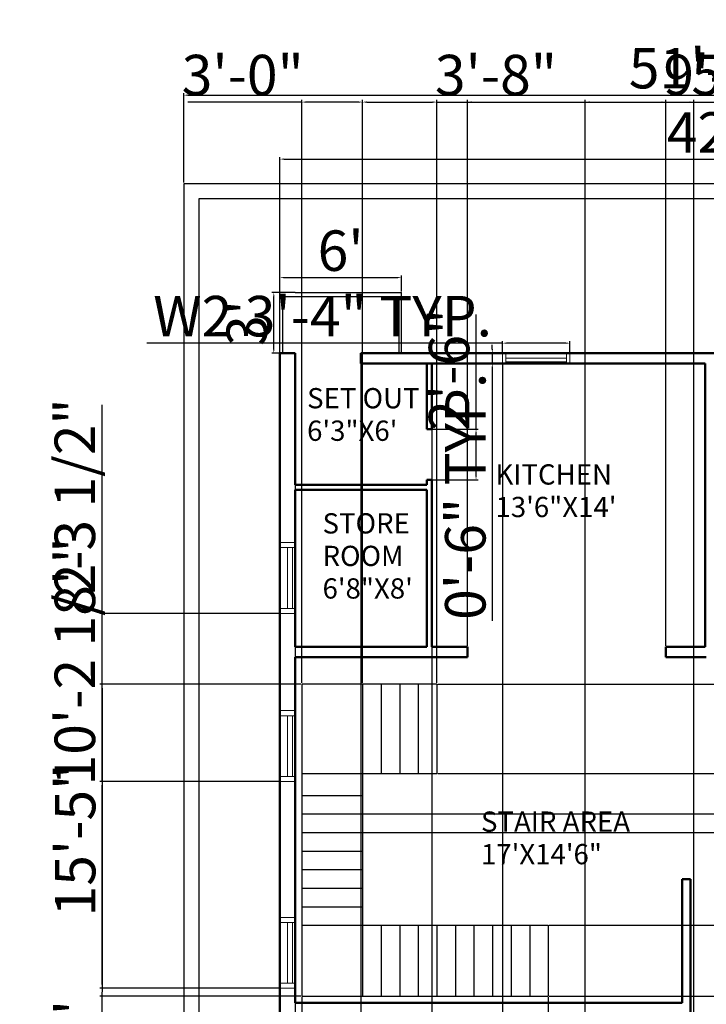
# Model space of a CAD drawing. Units: inches. Extents: x 2047 to 3023, y 479 to 1545.
# Tile 2 of 3: x 2047 to 2454, y 961 to 1545. Entities that reach past the tile are written whole.
import ezdxf

# ---------------------------------------------------------------- set-up
doc = ezdxf.new("R2010")
doc.units = ezdxf.units.IN
for name, color, linetype, lineweight in [('A-ANNO-DIMS', 2, 'Continuous', 18), ('A-AREA-IDEN', 7, 'Continuous', 25), ('A-FLOR', 8, 'Continuous', 25), ('A-FLOR-STRS', 7, 'Continuous', 25), ('A-GLAZ', 4, 'Continuous', 18), ('A-WALL', 7, 'Continuous', 50), ('C-PROP', 8, 'Continuous', 30)]:
    doc.layers.add(name, color=color, linetype=linetype, lineweight=lineweight)
doc.styles.get("Standard").update_dxf_attribs({"font": 'arial.ttf'})
doc.dimstyles.new('ISO-25', dxfattribs={"dimtxt": 24, "dimasz": 2.5, "dimexe": 1.25, "dimexo": 0.625, "dimtad": 1, "dimdec": 1, "dimlunit": 3, "dimtxsty": 'Standard', "dimcen": 2.5, "dimadec": 0, "dimazin": 0, "dimtfac": 1, "dimtdec": 1, "dimtmove": 0, "dimatfit": 3, "dimfxl": 1, "dimarcsym": 0})

# ---------------------------------------------------------------- blocks, each defined once
blk = doc.blocks.new('*D1')
at = {"layer": 'A-ANNO-DIMS', "color": 0, "lineweight": -2, "transparency": 16777216}
for p, q in [((2200.28, 1382.98), (2196.04, 1382.98)), ((2197.29, 1349.48), (2197.29, 1380.48)), ((2200.28, 1346.98), (2196.04, 1346.98))]:
    blk.add_line(p, q, dxfattribs=at)
at = {"layer": 'A-ANNO-DIMS', "color": 0, "transparency": 16777216}
for points in [[(2196.87, 1380.48), (2197.7, 1380.48), (2197.29, 1382.98)], [(2196.87, 1349.48), (2197.7, 1349.48), (2197.29, 1346.98)]]:
    blk.add_solid(points, dxfattribs=at)
at = {"layer": 'Defpoints', "color": 0, "transparency": 16777216}
for p in [(2197.29, 1382.98), (2200.91, 1382.98), (2200.91, 1346.98)]:
    blk.add_point(p, dxfattribs=at)
at = {"layer": 'A-ANNO-DIMS', "color": 0, "transparency": 16777216, "insert": (2184.4, 1364.98), "char_height": 24, "attachment_point": 5, "rotation": 90}
blk.add_mtext("3'", dxfattribs=at)
blk = doc.blocks.new('*D2')
at = {"layer": 'A-ANNO-DIMS', "color": 0, "lineweight": -2, "transparency": 16777216}
for p, q in [((2200.91, 1383.61), (2200.91, 1393.05)), ((2203.41, 1391.8), (2270.41, 1391.8)), ((2272.91, 1383.61), (2272.91, 1393.05))]:
    blk.add_line(p, q, dxfattribs=at)
at = {"layer": 'A-ANNO-DIMS', "color": 0, "transparency": 16777216}
for points in [[(2203.41, 1392.22), (2203.41, 1391.39), (2200.91, 1391.8)], [(2270.41, 1392.22), (2270.41, 1391.39), (2272.91, 1391.8)]]:
    blk.add_solid(points, dxfattribs=at)
at = {"layer": 'Defpoints', "color": 0, "transparency": 16777216}
for p in [(2272.91, 1391.8), (2200.91, 1382.98), (2272.91, 1382.98)]:
    blk.add_point(p, dxfattribs=at)
at = {"layer": 'A-ANNO-DIMS', "color": 0, "transparency": 16777216, "insert": (2236.91, 1404.68), "char_height": 24, "attachment_point": 5}
blk.add_mtext("6'", dxfattribs=at)
blk = doc.blocks.new('*D4')
at = {"layer": 'A-ANNO-DIMS', "color": 0, "lineweight": -2, "transparency": 16777216}
for p, q in [((2143.91, 1448.11), (2143.91, 1501.19)), ((2146.41, 1499.94), (2759.41, 1499.94)), ((2761.91, 1448.11), (2761.91, 1501.19))]:
    blk.add_line(p, q, dxfattribs=at)
at = {"layer": 'A-ANNO-DIMS', "color": 0, "transparency": 16777216}
for points in [[(2146.41, 1500.36), (2146.41, 1499.52), (2143.91, 1499.94)], [(2759.41, 1500.36), (2759.41, 1499.52), (2761.91, 1499.94)]]:
    blk.add_solid(points, dxfattribs=at)
at = {"layer": 'Defpoints', "color": 0, "transparency": 16777216}
for p in [(2761.91, 1499.94), (2143.91, 1447.48), (2761.91, 1447.48)]:
    blk.add_point(p, dxfattribs=at)
at = {"layer": 'A-ANNO-DIMS', "color": 0, "transparency": 16777216, "insert": (2452.91, 1512.82), "char_height": 24, "attachment_point": 5}
blk.add_mtext('51\'-6"', dxfattribs=at)
blk = doc.blocks.new('*D5')
at = {"layer": 'A-ANNO-DIMS', "color": 0, "lineweight": -2, "transparency": 16777216}
for p, q in [((2200.91, 1347.61), (2200.91, 1463.28)), ((2203.41, 1462.03), (2702.41, 1462.03)), ((2704.91, 1347.61), (2704.91, 1463.28))]:
    blk.add_line(p, q, dxfattribs=at)
at = {"layer": 'A-ANNO-DIMS', "color": 0, "transparency": 16777216}
for points in [[(2203.41, 1462.44), (2203.41, 1461.61), (2200.91, 1462.03)], [(2702.41, 1462.44), (2702.41, 1461.61), (2704.91, 1462.03)]]:
    blk.add_solid(points, dxfattribs=at)
at = {"layer": 'Defpoints', "color": 0, "transparency": 16777216}
for p in [(2704.91, 1462.03), (2200.91, 1346.98), (2704.91, 1346.98)]:
    blk.add_point(p, dxfattribs=at)
at = {"layer": 'A-ANNO-DIMS', "color": 0, "transparency": 16777216, "insert": (2452.91, 1474.7), "char_height": 24, "attachment_point": 5}
blk.add_mtext("42'", dxfattribs=at)
blk = doc.blocks.new('*D10')
at = {"layer": 'A-ANNO-DIMS', "color": 0, "lineweight": -2, "transparency": 16777216}
for p, q in [((2317.13, 1301.98), (2317.13, 1369.94)), ((2291.53, 1301.98), (2318.38, 1301.98)), ((2317.13, 1274.48), (2317.13, 1299.48)), ((2291.53, 1271.98), (2318.38, 1271.98))]:
    blk.add_line(p, q, dxfattribs=at)
at = {"layer": 'A-ANNO-DIMS', "color": 0, "transparency": 16777216}
for points in [[(2316.71, 1299.48), (2317.55, 1299.48), (2317.13, 1301.98)], [(2316.71, 1274.48), (2317.55, 1274.48), (2317.13, 1271.98)]]:
    blk.add_solid(points, dxfattribs=at)
at = {"layer": 'Defpoints', "color": 0, "transparency": 16777216}
for p in [(2290.91, 1301.98), (2317.13, 1301.98), (2290.91, 1271.98)]:
    blk.add_point(p, dxfattribs=at)
at = {"layer": 'A-ANNO-DIMS', "color": 0, "transparency": 16777216, "insert": (2304.25, 1337.21), "char_height": 24, "attachment_point": 5, "rotation": 90}
blk.add_mtext('2\'-6"', dxfattribs=at)
blk = doc.blocks.new('WIN-36IN-9IN-FRAME')
for p, q in [((9, 42), (0, 42)), ((9, 39), (0, 39)), ((0, 39), (0, 3)), ((4.5, 3), (4.5, 39)), ((7.5, 3), (7.5, 39)), ((9, 3), (9, 39)), ((0, 3), (9, 3)), ((0, 0), (9, 0))]:
    blk.add_line(p, q)
blk = doc.blocks.new('WIN-36IN-6IN-FRAME')
for p, q in [((0, 6), (0, 0)), ((38, 6), (2, 6)), ((2, 6), (2, 0)), ((38, 0), (38, 6)), ((40, 0), (40, 6)), ((38, 5), (2, 5)), ((38, 3), (2, 3)), ((2, 0), (38, 0))]:
    blk.add_line(p, q)
blk = doc.blocks.new('*D16')
at = {"layer": 'A-ANNO-DIMS', "color": 0, "lineweight": -2, "transparency": 16777216}
for p, q in [((2332.76, 1347.61), (2332.76, 1354.23)), ((2372.76, 1347.61), (2372.76, 1354.23)), ((2332.76, 1352.98), (2122.13, 1352.98)), ((2370.26, 1352.98), (2335.26, 1352.98))]:
    blk.add_line(p, q, dxfattribs=at)
at = {"layer": 'A-ANNO-DIMS', "color": 0, "transparency": 16777216}
for points in [[(2335.26, 1353.4), (2335.26, 1352.56), (2332.76, 1352.98)], [(2370.26, 1353.4), (2370.26, 1352.56), (2372.76, 1352.98)]]:
    blk.add_solid(points, dxfattribs=at)
at = {"layer": 'Defpoints', "color": 0, "transparency": 16777216}
for p in [(2332.76, 1352.98), (2332.76, 1346.98), (2372.76, 1346.98)]:
    blk.add_point(p, dxfattribs=at)
at = {"layer": 'A-ANNO-DIMS', "color": 0, "transparency": 16777216, "insert": (2226.2, 1365.87), "char_height": 24, "attachment_point": 5}
blk.add_mtext('W2 3\'-4" TYP.', dxfattribs=at)
blk = doc.blocks.new('*D17')
at = {"layer": 'A-ANNO-DIMS', "color": 0, "lineweight": -2, "transparency": 16777216}
for p, q in [((2326.76, 1349.48), (2326.76, 1351.98)), ((2332.14, 1346.98), (2325.51, 1346.98)), ((2326.76, 1346.98), (2326.76, 1340.98)), ((2332.14, 1340.98), (2325.51, 1340.98)), ((2326.76, 1338.48), (2326.76, 1188.44))]:
    blk.add_line(p, q, dxfattribs=at)
at = {"layer": 'A-ANNO-DIMS', "color": 0, "transparency": 16777216}
for points in [[(2326.35, 1349.48), (2327.18, 1349.48), (2326.76, 1346.98)], [(2326.35, 1338.48), (2327.18, 1338.48), (2326.76, 1340.98)]]:
    blk.add_solid(points, dxfattribs=at)
at = {"layer": 'Defpoints', "color": 0, "transparency": 16777216}
for p in [(2332.76, 1346.98), (2326.76, 1340.98), (2332.76, 1340.98)]:
    blk.add_point(p, dxfattribs=at)
at = {"layer": 'A-ANNO-DIMS', "color": 0, "transparency": 16777216, "insert": (2313.88, 1262.21), "char_height": 24, "attachment_point": 5, "rotation": 90}
blk.add_mtext('0\'-6" TYP.', dxfattribs=at)
blk = doc.blocks.new('*D29')
at = {"layer": 'A-ANNO-DIMS', "color": 0, "lineweight": -2, "transparency": 16777216}
for p, q in [((2200.28, 970.66), (2094.31, 970.66)), ((2095.56, 887.12), (2095.56, 968.16)), ((2200.28, 884.62), (2094.31, 884.62))]:
    blk.add_line(p, q, dxfattribs=at)
at = {"layer": 'A-ANNO-DIMS', "color": 0, "transparency": 16777216}
for points in [[(2095.14, 968.16), (2095.97, 968.16), (2095.56, 970.66)], [(2095.14, 887.12), (2095.97, 887.12), (2095.56, 884.62)]]:
    blk.add_solid(points, dxfattribs=at)
at = {"layer": 'Defpoints', "color": 0, "transparency": 16777216}
for p in [(2095.56, 970.66), (2200.91, 970.66), (2200.91, 884.62)]:
    blk.add_point(p, dxfattribs=at)
at = {"layer": 'A-ANNO-DIMS', "color": 0, "transparency": 16777216, "insert": (2082.88, 927.64), "char_height": 24, "attachment_point": 5, "rotation": 90}
blk.add_mtext('7\'-2"', dxfattribs=at)
blk = doc.blocks.new('*D30')
at = {"layer": 'A-ANNO-DIMS', "color": 0, "lineweight": -2, "transparency": 16777216}
for p, q in [((2095.56, 1093.2), (2095.56, 1233.06)), ((2200.28, 1093.2), (2094.31, 1093.2)), ((2095.56, 973.16), (2095.56, 1090.7)), ((2200.28, 970.66), (2094.31, 970.66))]:
    blk.add_line(p, q, dxfattribs=at)
at = {"layer": 'A-ANNO-DIMS', "color": 0, "transparency": 16777216}
for points in [[(2095.14, 1090.7), (2095.97, 1090.7), (2095.56, 1093.2)], [(2095.14, 973.16), (2095.97, 973.16), (2095.56, 970.66)]]:
    blk.add_solid(points, dxfattribs=at)
at = {"layer": 'Defpoints', "color": 0, "transparency": 16777216}
for p in [(2095.56, 1093.2), (2200.91, 1093.2), (2200.91, 970.66)]:
    blk.add_point(p, dxfattribs=at)
at = {"layer": 'A-ANNO-DIMS', "color": 0, "transparency": 16777216, "insert": (2082.52, 1164.38), "char_height": 24, "attachment_point": 5, "rotation": 90}
blk.add_mtext('10\'-2 1/2"', dxfattribs=at)
blk = doc.blocks.new('*D31')
at = {"layer": 'A-ANNO-DIMS', "color": 0, "lineweight": -2, "transparency": 16777216}
for p, q in [((2095.56, 1192.82), (2095.56, 1316.32)), ((2200.28, 1192.82), (2094.31, 1192.82)), ((2095.56, 1095.7), (2095.56, 1190.32)), ((2200.28, 1093.2), (2094.31, 1093.2))]:
    blk.add_line(p, q, dxfattribs=at)
at = {"layer": 'A-ANNO-DIMS', "color": 0, "transparency": 16777216}
for points in [[(2095.14, 1190.32), (2095.97, 1190.32), (2095.56, 1192.82)], [(2095.14, 1095.7), (2095.97, 1095.7), (2095.56, 1093.2)]]:
    blk.add_solid(points, dxfattribs=at)
at = {"layer": 'Defpoints', "color": 0, "transparency": 16777216}
for p in [(2095.56, 1192.82), (2200.91, 1192.82), (2200.91, 1093.2)]:
    blk.add_point(p, dxfattribs=at)
at = {"layer": 'A-ANNO-DIMS', "color": 0, "transparency": 16777216, "insert": (2082.52, 1255.82), "char_height": 24, "attachment_point": 5, "rotation": 90}
blk.add_mtext('8\'-3 1/2"', dxfattribs=at)
blk = doc.blocks.new('*D37')
at = {"layer": 'A-ANNO-DIMS', "color": 0, "lineweight": -2, "transparency": 16777216}
for p, q in [((2290.91, 1340.36), (2290.91, 500.88)), ((2332.76, 1340.36), (2332.76, 500.88)), ((2293.41, 502.13), (2330.26, 502.13)), ((2332.76, 502.13), (2400.29, 502.13))]:
    blk.add_line(p, q, dxfattribs=at)
at = {"layer": 'A-ANNO-DIMS', "color": 0, "transparency": 16777216}
for points in [[(2293.41, 502.55), (2293.41, 501.71), (2290.91, 502.13)], [(2330.26, 502.55), (2330.26, 501.71), (2332.76, 502.13)]]:
    blk.add_solid(points, dxfattribs=at)
at = {"layer": 'Defpoints', "color": 0, "transparency": 16777216}
for p in [(2290.91, 1340.98), (2332.76, 1340.98), (2332.76, 502.13)]:
    blk.add_point(p, dxfattribs=at)
at = {"layer": 'A-ANNO-DIMS', "color": 0, "transparency": 16777216, "insert": (2367.78, 515.02), "char_height": 24, "attachment_point": 5}
blk.add_mtext('3\'-6"', dxfattribs=at)
blk = doc.blocks.new('*D41')
at = {"layer": 'A-ANNO-DIMS', "color": 0, "lineweight": -2, "transparency": 16777216}
for p, q in [((2381.88, 867.61), (2381.88, 1497.08)), ((2384.38, 1495.83), (2443.66, 1495.83)), ((2446.16, 867.61), (2446.16, 1497.08)), ((2446.16, 1495.83), (2569.64, 1495.83))]:
    blk.add_line(p, q, dxfattribs=at)
at = {"layer": 'A-ANNO-DIMS', "color": 0, "transparency": 16777216}
for points in [[(2384.38, 1496.25), (2384.38, 1495.41), (2381.88, 1495.83)], [(2443.66, 1496.25), (2443.66, 1495.41), (2446.16, 1495.83)]]:
    blk.add_solid(points, dxfattribs=at)
at = {"layer": 'Defpoints', "color": 0, "transparency": 16777216}
for p in [(2446.16, 1495.83), (2381.88, 866.98), (2446.16, 866.98)]:
    blk.add_point(p, dxfattribs=at)
at = {"layer": 'A-ANNO-DIMS', "color": 0, "transparency": 16777216, "insert": (2509.15, 1508.86), "char_height": 24, "attachment_point": 5}
blk.add_mtext('5\'-4 1/2"', dxfattribs=at)
blk = doc.blocks.new('*D42')
at = {"layer": 'A-ANNO-DIMS', "color": 0, "lineweight": -2, "transparency": 16777216}
for p, q in [((2810.26, 950.97), (2810.26, 1016.25)), ((2362.53, 950.97), (2811.51, 950.97)), ((2810.26, 932.42), (2810.26, 948.47)), ((2362.53, 929.92), (2811.51, 929.92))]:
    blk.add_line(p, q, dxfattribs=at)
at = {"layer": 'A-ANNO-DIMS', "color": 0, "transparency": 16777216}
for points in [[(2809.84, 948.47), (2810.67, 948.47), (2810.26, 950.97)], [(2809.84, 932.42), (2810.67, 932.42), (2810.26, 929.92)]]:
    blk.add_solid(points, dxfattribs=at)
at = {"layer": 'Defpoints', "color": 0, "transparency": 16777216}
for p in [(2361.91, 950.97), (2810.26, 950.97), (2361.91, 929.92)]:
    blk.add_point(p, dxfattribs=at)
at = {"layer": 'A-ANNO-DIMS', "color": 0, "transparency": 16777216, "insert": (2797.38, 984.86), "char_height": 24, "attachment_point": 5, "rotation": 90}
blk.add_mtext('1\'-9"', dxfattribs=at)
blk = doc.blocks.new('*D43')
at = {"layer": 'A-ANNO-DIMS', "color": 0, "lineweight": -2, "transparency": 16777216}
for p, q in [((2213.91, 965.36), (2213.91, 500.88)), ((2359.91, 965.36), (2359.91, 500.88)), ((2216.41, 502.13), (2357.41, 502.13))]:
    blk.add_line(p, q, dxfattribs=at)
at = {"layer": 'A-ANNO-DIMS', "color": 0, "transparency": 16777216}
for points in [[(2216.41, 502.55), (2216.41, 501.71), (2213.91, 502.13)], [(2357.41, 502.55), (2357.41, 501.71), (2359.91, 502.13)]]:
    blk.add_solid(points, dxfattribs=at)
at = {"layer": 'Defpoints', "color": 0, "transparency": 16777216}
for p in [(2213.91, 965.98), (2359.91, 965.98), (2359.91, 502.13)]:
    blk.add_point(p, dxfattribs=at)
at = {"layer": 'A-ANNO-DIMS', "color": 0, "transparency": 16777216, "insert": (2286.91, 514.8), "char_height": 24, "attachment_point": 5}
blk.add_mtext('12\'-2"', dxfattribs=at)
blk = doc.blocks.new('*D44')
at = {"layer": 'A-ANNO-DIMS', "color": 0, "lineweight": -2, "transparency": 16777216}
for p, q in [((2213.28, 1150.98), (2094.31, 1150.98)), ((2095.56, 1148.48), (2095.56, 968.48)), ((2213.28, 965.98), (2094.31, 965.98))]:
    blk.add_line(p, q, dxfattribs=at)
at = {"layer": 'A-ANNO-DIMS', "color": 0, "transparency": 16777216}
for points in [[(2095.14, 1148.48), (2095.97, 1148.48), (2095.56, 1150.98)], [(2095.14, 968.48), (2095.97, 968.48), (2095.56, 965.98)]]:
    blk.add_solid(points, dxfattribs=at)
at = {"layer": 'Defpoints', "color": 0, "transparency": 16777216}
for p in [(2213.91, 1150.98), (2095.56, 965.98), (2213.91, 965.98)]:
    blk.add_point(p, dxfattribs=at)
at = {"layer": 'A-ANNO-DIMS', "color": 0, "transparency": 16777216, "insert": (2082.68, 1058.48), "char_height": 24, "attachment_point": 5, "rotation": 90}
blk.add_mtext('15\'-5"', dxfattribs=at)
blk = doc.blocks.new('*D45')
at = {"layer": 'A-ANNO-DIMS', "color": 0, "lineweight": -2, "transparency": 16777216}
for p, q in [((2213.91, 1495.83), (2146.38, 1495.83)), ((2213.91, 1151.61), (2213.91, 1497.08)), ((2247.41, 1495.83), (2216.41, 1495.83)), ((2249.91, 1151.61), (2249.91, 1497.08))]:
    blk.add_line(p, q, dxfattribs=at)
at = {"layer": 'A-ANNO-DIMS', "color": 0, "transparency": 16777216}
for points in [[(2216.41, 1496.25), (2216.41, 1495.41), (2213.91, 1495.83)], [(2247.41, 1496.25), (2247.41, 1495.41), (2249.91, 1495.83)]]:
    blk.add_solid(points, dxfattribs=at)
at = {"layer": 'Defpoints', "color": 0, "transparency": 16777216}
for p in [(2213.91, 1495.83), (2213.91, 1150.98), (2249.91, 1150.98)]:
    blk.add_point(p, dxfattribs=at)
at = {"layer": 'A-ANNO-DIMS', "color": 0, "transparency": 16777216, "insert": (2178.89, 1508.72), "char_height": 24, "attachment_point": 5}
blk.add_mtext('3\'-0"', dxfattribs=at)
blk = doc.blocks.new('*D46')
at = {"layer": 'A-ANNO-DIMS', "color": 0, "lineweight": -2, "transparency": 16777216}
for p, q in [((2810.26, 1007.98), (2810.26, 1075.51)), ((2360.53, 1007.98), (2811.51, 1007.98)), ((2810.26, 968.48), (2810.26, 1005.48)), ((2360.53, 965.98), (2811.51, 965.98))]:
    blk.add_line(p, q, dxfattribs=at)
at = {"layer": 'A-ANNO-DIMS', "color": 0, "transparency": 16777216}
for points in [[(2809.84, 1005.48), (2810.67, 1005.48), (2810.26, 1007.98)], [(2809.84, 968.48), (2810.67, 968.48), (2810.26, 965.98)]]:
    blk.add_solid(points, dxfattribs=at)
at = {"layer": 'Defpoints', "color": 0, "transparency": 16777216}
for p in [(2359.91, 1007.98), (2810.26, 1007.98), (2359.91, 965.98)]:
    blk.add_point(p, dxfattribs=at)
at = {"layer": 'A-ANNO-DIMS', "color": 0, "transparency": 16777216, "insert": (2797.37, 1043), "char_height": 24, "attachment_point": 5, "rotation": 90}
blk.add_mtext('3\'-6"', dxfattribs=at)
blk = doc.blocks.new('*D47')
at = {"layer": 'A-ANNO-DIMS', "color": 0, "lineweight": -2, "transparency": 16777216}
for p, q in [((2810.26, 1150.98), (2810.26, 1219.49)), ((2294.53, 1150.98), (2811.51, 1150.98)), ((2810.26, 1100.48), (2810.26, 1148.48)), ((2294.53, 1097.98), (2811.51, 1097.98))]:
    blk.add_line(p, q, dxfattribs=at)
at = {"layer": 'A-ANNO-DIMS', "color": 0, "transparency": 16777216}
for points in [[(2809.84, 1148.48), (2810.67, 1148.48), (2810.26, 1150.98)], [(2809.84, 1100.48), (2810.67, 1100.48), (2810.26, 1097.98)]]:
    blk.add_solid(points, dxfattribs=at)
at = {"layer": 'Defpoints', "color": 0, "transparency": 16777216}
for p in [(2293.91, 1150.98), (2810.26, 1150.98), (2293.91, 1097.98)]:
    blk.add_point(p, dxfattribs=at)
at = {"layer": 'A-ANNO-DIMS', "color": 0, "transparency": 16777216, "insert": (2797.43, 1186.49), "char_height": 24, "attachment_point": 5, "rotation": 90}
blk.add_mtext('4\'-5"', dxfattribs=at)
blk = doc.blocks.new('*D48')
at = {"layer": 'A-ANNO-DIMS', "color": 0, "lineweight": -2, "transparency": 16777216}
for p, q in [((2249.91, 1151.61), (2249.91, 1497.08)), ((2252.41, 1495.83), (2291.41, 1495.83)), ((2293.91, 1151.61), (2293.91, 1497.08)), ((2293.91, 1495.83), (2361.44, 1495.83))]:
    blk.add_line(p, q, dxfattribs=at)
at = {"layer": 'A-ANNO-DIMS', "color": 0, "transparency": 16777216}
for points in [[(2252.41, 1496.25), (2252.41, 1495.41), (2249.91, 1495.83)], [(2291.41, 1496.25), (2291.41, 1495.41), (2293.91, 1495.83)]]:
    blk.add_solid(points, dxfattribs=at)
at = {"layer": 'Defpoints', "color": 0, "transparency": 16777216}
for p in [(2293.91, 1495.83), (2249.91, 1150.98), (2293.91, 1150.98)]:
    blk.add_point(p, dxfattribs=at)
at = {"layer": 'A-ANNO-DIMS', "color": 0, "transparency": 16777216, "insert": (2328.92, 1508.72), "char_height": 24, "attachment_point": 5}
blk.add_mtext('3\'-8"', dxfattribs=at)
blk = doc.blocks.new('*D49')
at = {"layer": 'A-ANNO-DIMS', "color": 0, "lineweight": -2, "transparency": 16777216}
for p, q in [((2250.53, 1073.98), (2811.51, 1073.98)), ((2810.26, 1071.48), (2810.26, 1065.48)), ((2250.53, 1062.98), (2811.51, 1062.98)), ((2810.26, 1062.98), (2810.26, 976.79))]:
    blk.add_line(p, q, dxfattribs=at)
at = {"layer": 'A-ANNO-DIMS', "color": 0, "transparency": 16777216}
for points in [[(2809.84, 1071.48), (2810.67, 1071.48), (2810.26, 1073.98)], [(2809.84, 1065.48), (2810.67, 1065.48), (2810.26, 1062.98)]]:
    blk.add_solid(points, dxfattribs=at)
at = {"layer": 'Defpoints', "color": 0, "transparency": 16777216}
for p in [(2249.91, 1073.98), (2249.91, 1062.98), (2810.26, 1062.98)]:
    blk.add_point(p, dxfattribs=at)
at = {"layer": 'A-ANNO-DIMS', "color": 0, "transparency": 16777216, "insert": (2797.38, 1018.63), "char_height": 24, "attachment_point": 5, "rotation": 90}
blk.add_mtext('0\'-11"', dxfattribs=at)
blk = doc.blocks.new('*D50')
at = {"layer": 'A-ANNO-DIMS', "color": 0, "lineweight": -2, "transparency": 16777216}
for p, q in [((2311.99, 1173.61), (2311.99, 1497.08)), ((2314.49, 1495.83), (2427.04, 1495.83)), ((2429.54, 1173.61), (2429.54, 1497.08)), ((2429.54, 1495.83), (2553.01, 1495.83))]:
    blk.add_line(p, q, dxfattribs=at)
at = {"layer": 'A-ANNO-DIMS', "color": 0, "transparency": 16777216}
for points in [[(2314.49, 1496.25), (2314.49, 1495.41), (2311.99, 1495.83)], [(2427.04, 1496.25), (2427.04, 1495.41), (2429.54, 1495.83)]]:
    blk.add_solid(points, dxfattribs=at)
at = {"layer": 'Defpoints', "color": 0, "transparency": 16777216}
for p in [(2429.54, 1495.83), (2311.99, 1172.98), (2429.54, 1172.98)]:
    blk.add_point(p, dxfattribs=at)
at = {"layer": 'A-ANNO-DIMS', "color": 0, "transparency": 16777216, "insert": (2492.53, 1508.86), "char_height": 24, "attachment_point": 5}
blk.add_mtext('9\'-9 1/2"', dxfattribs=at)
blk = doc.blocks.new('*D53')
at = {"layer": 'A-ANNO-DIMS', "color": 0, "lineweight": -2, "transparency": 16777216}
for p, q in [((2209.91, 1346.36), (2209.91, 500.88)), ((2248.87, 1346.36), (2248.87, 500.88)), ((2212.41, 502.13), (2246.37, 502.13)), ((2248.87, 502.13), (2316.4, 502.13))]:
    blk.add_line(p, q, dxfattribs=at)
at = {"layer": 'A-ANNO-DIMS', "color": 0, "transparency": 16777216}
for points in [[(2212.41, 502.55), (2212.41, 501.71), (2209.91, 502.13)], [(2246.37, 502.55), (2246.37, 501.71), (2248.87, 502.13)]]:
    blk.add_solid(points, dxfattribs=at)
at = {"layer": 'Defpoints', "color": 0, "transparency": 16777216}
for p in [(2209.91, 1346.98), (2248.87, 1346.98), (2248.87, 502.13)]:
    blk.add_point(p, dxfattribs=at)
at = {"layer": 'A-ANNO-DIMS', "color": 0, "transparency": 16777216, "insert": (2283.89, 515.02), "char_height": 24, "attachment_point": 5}
blk.add_mtext('3\'-3"', dxfattribs=at)

msp = doc.modelspace()

# ---------------------------------------------------------------- linework, layer by layer
at = {"layer": 'A-FLOR'}
for p, q in [((2209.91, 1382.98), (2200.91, 1382.98)), ((2200.91, 1346.98), (2200.91, 1382.98)), ((2209.91, 1382.98), (2272.91, 1382.98)), ((2272.91, 1346.98), (2272.91, 1382.98)), ((2202.71, 1346.98), (2202.71, 1380.63)), ((2202.71, 1380.63), (2271.36, 1380.63)), ((2271.36, 1380.63), (2271.36, 1346.98))]:
    msp.add_line(p, q, dxfattribs=at)
at = {"layer": 'A-FLOR-STRS'}
for p, q in [((2213.91, 1150.98), (2213.91, 965.98)), ((2293.91, 1150.98), (2213.91, 1150.98)), ((2249.91, 1150.98), (2249.91, 965.98)), ((2260.91, 1150.98), (2260.91, 1097.98)), ((2271.91, 1150.98), (2271.91, 1097.98)), ((2282.91, 1150.98), (2282.91, 1097.98)), ((2293.91, 1150.98), (2293.91, 1097.98)), ((2213.91, 1097.98), (2293.91, 1097.98)), ((2213.91, 1084.98), (2249.91, 1084.98)), ((2213.91, 1073.98), (2249.91, 1073.98)), ((2213.91, 1062.98), (2249.91, 1062.98)), ((2213.91, 1051.98), (2249.91, 1051.98)), ((2213.91, 1040.98), (2249.91, 1040.98)), ((2213.91, 1029.98), (2249.91, 1029.98)), ((2213.91, 1018.98), (2249.91, 1018.98)), ((2213.91, 1007.98), (2359.91, 1007.98)), ((2260.91, 1007.98), (2260.91, 965.98)), ((2271.91, 1007.98), (2271.91, 965.98)), ((2282.91, 1007.98), (2282.91, 965.98)), ((2293.91, 1007.98), (2293.91, 965.98)), ((2304.91, 1007.98), (2304.91, 965.98)), ((2315.91, 1007.98), (2315.91, 965.98)), ((2326.91, 1007.98), (2326.91, 965.98)), ((2337.91, 1007.98), (2337.91, 965.98)), ((2348.91, 1007.98), (2348.91, 965.98)), ((2359.91, 1007.98), (2359.91, 965.98)), ((2213.91, 965.98), (2359.91, 965.98))]:
    msp.add_line(p, q, dxfattribs=at)
at = {"layer": 'A-WALL'}
for p, q in [((2200.91, 1346.98), (2200.91, 650.98)), ((2209.91, 1346.98), (2200.91, 1346.98)), ((2209.91, 1346.98), (2209.91, 1268.98)), ((2704.91, 1346.98), (2248.87, 1346.98)), ((2248.87, 1346.98), (2248.87, 1340.98)), ((2452.91, 1340.98), (2248.87, 1340.98)), ((2287.91, 1301.98), (2287.91, 1340.98)), ((2290.91, 1301.98), (2290.91, 1340.98)), ((2452.91, 1172.98), (2452.91, 1340.98)), ((2287.91, 1301.98), (2290.91, 1301.98)), ((2287.91, 1268.98), (2209.91, 1268.98)), ((2287.91, 1268.98), (2287.91, 1271.98)), ((2287.91, 1271.98), (2290.91, 1271.98)), ((2290.91, 1172.98), (2290.91, 1271.98)), ((2287.91, 1265.98), (2209.91, 1265.98)), ((2209.91, 1265.98), (2209.91, 1172.98)), ((2287.91, 1172.98), (2287.91, 1265.98)), ((2287.91, 1172.98), (2209.91, 1172.98)), ((2311.99, 1172.98), (2290.91, 1172.98)), ((2311.99, 1166.98), (2311.99, 1172.98)), ((2452.91, 1172.98), (2429.54, 1172.98)), ((2429.54, 1166.98), (2429.54, 1172.98)), ((2311.99, 1166.98), (2209.91, 1166.98)), ((2209.91, 1166.98), (2209.91, 961.98)), ((2452.91, 1166.98), (2429.54, 1166.98)), ((2453.57, 1166.97), (2452.91, 1166.98)), ((2439.19, 1035.32), (2442.95, 1035.32)), ((2439.19, 961.98), (2439.19, 1035.32)), ((2442.95, 1035.32), (2444.25, 1035.32)), ((2444.25, 950.97), (2444.25, 1035.32)), ((2209.91, 961.98), (2361.91, 961.98)), ((2361.91, 961.98), (2439.19, 961.98))]:
    msp.add_line(p, q, dxfattribs=at)
at = {"layer": 'C-PROP'}
for points in [[(2692.81, 550.48), (2761.91, 550.48), (2761.91, 1447.48), (2143.91, 1447.48), (2143.91, 550.48), (2554.81, 550.48)], [(2692.81, 559.48), (2752.91, 559.48), (2752.91, 1438.48), (2152.91, 1438.48), (2152.91, 559.48), (2554.81, 559.48)]]:
    msp.add_lwpolyline(points, dxfattribs=at)

# ---------------------------------------------------------------- block references
at = {"layer": 'A-GLAZ', "rotation": 180}
msp.add_blockref('WIN-36IN-6IN-FRAME', (2372.76, 1346.98), dxfattribs=at)
at = {"layer": 'A-GLAZ'}
for p in [(2200.91, 1192.82), (2200.91, 1093.2), (2200.91, 970.66)]:
    msp.add_blockref('WIN-36IN-9IN-FRAME', p, dxfattribs=at)

# ---------------------------------------------------------------- texts
at = {"layer": 'A-AREA-IDEN'}
for s, p in [('SET OUT', (2217.03, 1314.35)), ('6\'3"X6\'', (2217.03, 1295.08)), ('KITCHEN', (2328.66, 1269.16)), ('13\'6"X14\'', (2328.66, 1249.89)), ('STORE', (2226.17, 1240.17)), ('ROOM', (2226.17, 1220.89)), ('6\'8"X8\'', (2226.17, 1201.61)), ('STAIR AREA', (2320.07, 1063.43)), ('17\'X14\'6"', (2320.07, 1044.15))]:
    msp.add_text(s, height=12, dxfattribs=at).set_placement(p)

# ---------------------------------------------------------------- dimensions: what is measured, and where the dimension line sits
at = {"layer": 'A-ANNO-DIMS'}
for base, p1, p2, override, picture, middle in [((2429.5398, 1495.8302), (2311.9877, 1172.9802), (2429.5398, 1172.9802), {"dimdec": 1, "dimlfac": 1, "dimrnd": 0, "dimzin": 1, "dimdsep": 46, "dimlunit": 4, "dimfrac": 2}, '*D50', (2492.5257, 1508.8645)), ((2446.16, 1495.83), (2381.88, 866.98), (2446.16, 866.98), {"dimdec": 1, "dimlfac": 1, "dimrnd": 0, "dimzin": 1, "dimdsep": 46, "dimlunit": 4, "dimfrac": 2}, '*D41', (2509.15, 1508.86)), ((2761.91, 1499.94), (2143.91, 1447.48), (2761.91, 1447.48), {"dimclrd": 0, "dimclre": 0, "dimclrt": 0}, '*D4', (2452.91, 1512.82)), ((2213.91, 1495.83), (2249.91, 1150.98), (2213.91, 1150.98), {"dimdec": 1, "dimlfac": 1, "dimrnd": 0, "dimzin": 1, "dimdsep": 46, "dimlunit": 4, "dimfrac": 2}, '*D45', (2178.89, 1508.72)), ((2293.91, 1495.83), (2249.91, 1150.98), (2293.91, 1150.98), {"dimdec": 1, "dimlfac": 1, "dimrnd": 0, "dimzin": 1, "dimdsep": 46, "dimlunit": 4, "dimfrac": 2}, '*D48', (2328.92, 1508.72)), ((2704.91, 1462.03), (2200.91, 1346.98), (2704.91, 1346.98), {"dimclrd": 0, "dimclre": 0, "dimclrt": 0}, '*D5', (2452.91, 1474.7)), ((2272.91, 1391.8), (2200.91, 1382.98), (2272.91, 1382.98), {"dimclrd": 0, "dimclre": 0, "dimclrt": 0}, '*D2', (2236.91, 1404.68)), ((2248.87, 502.13), (2209.91, 1346.98), (2248.87, 1346.98), {"dimdec": 1, "dimlfac": 1, "dimrnd": 0, "dimzin": 1, "dimdsep": 46, "dimlunit": 4, "dimfrac": 2}, '*D53', (2283.89, 515.02)), ((2332.7623, 502.1302), (2290.908, 1340.9802), (2332.7623, 1340.9802), {"dimdec": 1, "dimlfac": 1, "dimrnd": 0, "dimzin": 1, "dimdsep": 46, "dimlunit": 4, "dimfrac": 2}, '*D37', (2367.7782, 515.0172)), ((2359.91, 502.13), (2213.91, 965.98), (2359.91, 965.98), {"dimdec": 1, "dimlfac": 1, "dimrnd": 0, "dimzin": 1, "dimdsep": 46, "dimlunit": 4, "dimfrac": 2}, '*D43', (2286.91, 514.8))]:
    dim = msp.add_linear_dim(base=base, p1=p1, p2=p2, dimstyle='ISO-25', override=override, dxfattribs=at)
    dim.commit()
    dim.dimension.update_dxf_attribs({"geometry": picture, "text_midpoint": middle})
for base, p1, p2, angle, text, picture, middle in [((2332.76, 1352.98), (2372.76, 1346.98), (2332.76, 1346.98), 180, 'W2 <> TYP.', '*D16', (2226.2, 1365.87)), ((2326.76, 1340.98), (2332.76, 1346.98), (2332.76, 1340.98), 270, '<> TYP.', '*D17', (2313.88, 1262.21))]:
    dim = msp.add_linear_dim(base=base, p1=p1, p2=p2, angle=angle, text=text, dimstyle='ISO-25', override={"dimdec": 1, "dimlfac": 1, "dimrnd": 0, "dimzin": 1, "dimdsep": 46, "dimlunit": 4, "dimfrac": 2}, dxfattribs=at)
    dim.commit()
    dim.dimension.update_dxf_attribs({"geometry": picture, "text_midpoint": middle})
for base, p1, p2, override, picture, middle in [((2197.29, 1382.98), (2200.91, 1346.98), (2200.91, 1382.98), {"dimclrd": 0, "dimclre": 0, "dimclrt": 0}, '*D1', (2184.4, 1364.98)), ((2317.13, 1301.98), (2290.91, 1271.98), (2290.91, 1301.98), {"dimclrd": 0, "dimclre": 0, "dimclrt": 0}, '*D10', (2304.25, 1337.21)), ((2095.56, 1192.82), (2200.91, 1093.2), (2200.91, 1192.82), {"dimdec": 1, "dimlfac": 1, "dimrnd": 0, "dimzin": 1, "dimdsep": 46, "dimlunit": 4, "dimfrac": 2}, '*D31', (2082.52, 1255.82)), ((2095.56, 1093.2), (2200.91, 970.66), (2200.91, 1093.2), {"dimdec": 1, "dimlfac": 1, "dimrnd": 0, "dimzin": 1, "dimdsep": 46, "dimlunit": 4, "dimfrac": 2}, '*D30', (2082.52, 1164.38)), ((2810.26, 1150.98), (2293.91, 1097.98), (2293.91, 1150.98), {"dimdec": 1, "dimlfac": 1, "dimrnd": 0, "dimzin": 1, "dimdsep": 46, "dimlunit": 4, "dimfrac": 2}, '*D47', (2797.43, 1186.49)), ((2095.56, 965.98), (2213.91, 1150.98), (2213.91, 965.98), {"dimdec": 1, "dimlfac": 1, "dimrnd": 0, "dimzin": 1, "dimdsep": 46, "dimlunit": 4, "dimfrac": 2}, '*D44', (2082.68, 1058.48)), ((2810.26, 1062.98), (2249.91, 1073.98), (2249.91, 1062.98), {"dimdec": 1, "dimlfac": 1, "dimrnd": 0, "dimzin": 1, "dimdsep": 46, "dimlunit": 4, "dimfrac": 2}, '*D49', (2797.38, 1018.63)), ((2810.26, 1007.98), (2359.91, 965.98), (2359.91, 1007.98), {"dimdec": 1, "dimlfac": 1, "dimrnd": 0, "dimzin": 1, "dimdsep": 46, "dimlunit": 4, "dimfrac": 2}, '*D46', (2797.37, 1043)), ((2810.258, 950.966), (2361.908, 929.9219), (2361.908, 950.966), {"dimdec": 1, "dimlfac": 1, "dimrnd": 0, "dimzin": 1, "dimdsep": 46, "dimlunit": 4, "dimfrac": 2}, '*D42', (2797.3792, 984.8604)), ((2095.56, 970.66), (2200.91, 884.62), (2200.91, 970.66), {"dimdec": 1, "dimlfac": 1, "dimrnd": 0, "dimzin": 1, "dimdsep": 46, "dimlunit": 4, "dimfrac": 2}, '*D29', (2082.88, 927.64))]:
    dim = msp.add_linear_dim(base=base, p1=p1, p2=p2, angle=90, dimstyle='ISO-25', override=override, dxfattribs=at)
    dim.commit()
    dim.dimension.update_dxf_attribs({"geometry": picture, "text_midpoint": middle})

doc.saveas('drawing.dxf')
